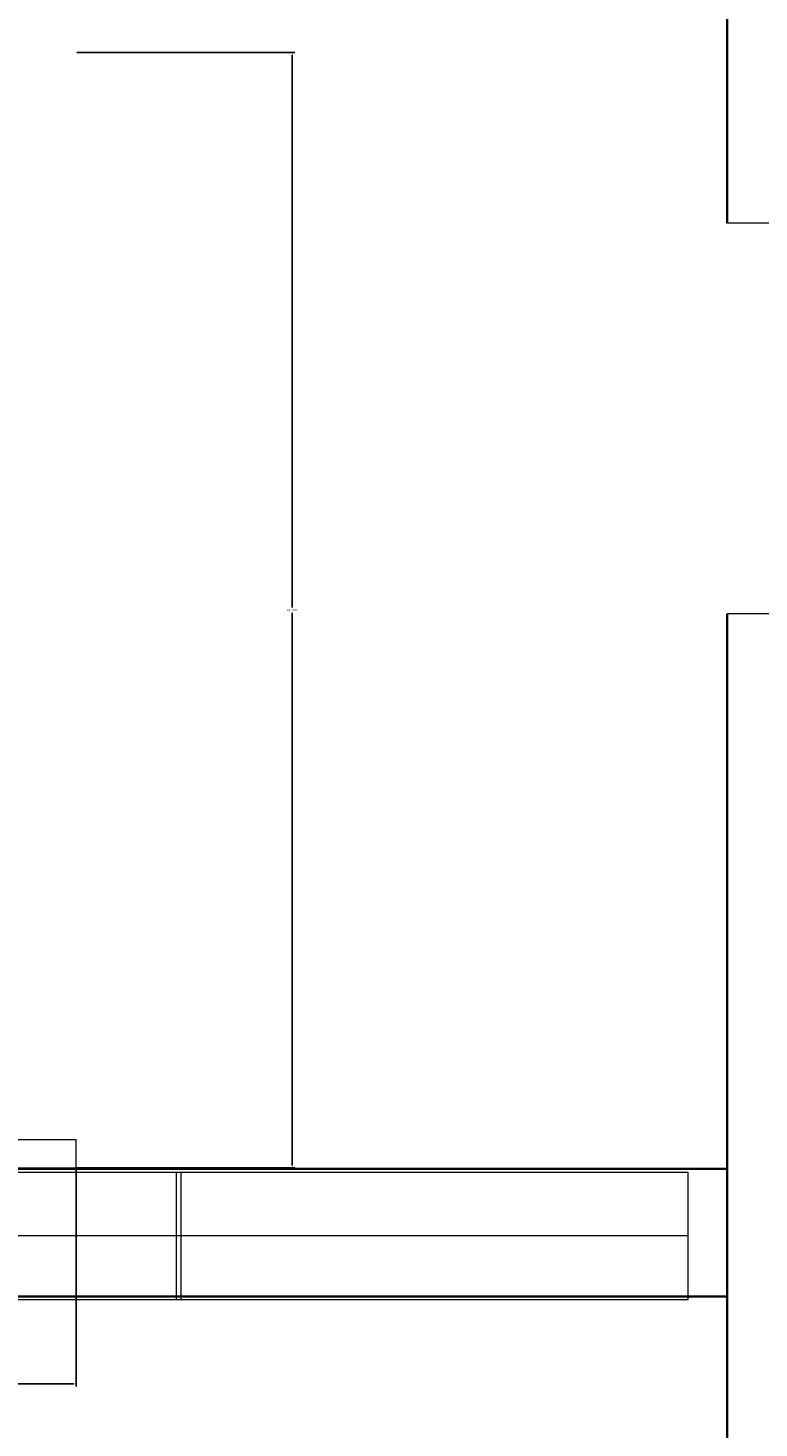
# Model space of a CAD drawing. Units: millimetres. Extents: x 27017497 to 27018854, y 7058029 to 7059154.
# Tile 27 of 91: x 27017753 to 27017804, y 7058124 to 7058222. Entities that reach past the tile are written whole.
import ezdxf

# ---------------------------------------------------------------- set-up
doc = ezdxf.new("R2010")
doc.units = ezdxf.units.MM
for name, color, linetype, lineweight in [('A-ANNO-DIMS', 2, 'Continuous', 18), ('A-DOOR', 4, 'Continuous', 20), ('A-FURN', 8, 'Continuous', 18), ('A-GLAZ', 4, 'Continuous', 18), ('A-WALL', 7, 'Continuous', 35)]:
    doc.layers.add(name, color=color, linetype=linetype, lineweight=lineweight)
doc.styles.get("Standard").update_dxf_attribs({"font": 'arial.ttf'})
doc.dimstyles.get("Standard").update_dxf_attribs({"dimtxt": 0.18, "dimasz": 0.18, "dimexe": 0.18, "dimexo": 0.0625, "dimgap": 0.09, "dimtad": 0, "dimtih": 1, "dimtoh": 1, "dimdec": 4, "dimzin": 0, "dimdsep": 46, "dimtxsty": 'Standard', "dimcen": 0.09, "dimadec": 0, "dimazin": 0, "dimtfac": 1, "dimtdec": 4, "dimtofl": 0, "dimtmove": 0, "dimatfit": 3, "dimfxl": 1, "dimtolj": 1, "dimtzin": 0, "dimarcsym": 0})

# ---------------------------------------------------------------- blocks, each defined once
blk = doc.blocks.new('*U2')
for p, q in [((0, 0), (0, -6)), ((40, 0), (40, -6))]:
    blk.add_line(p, q)
blk.add_lwpolyline([(0, 0), (0, 40), (1.75, 40), (1.75, 0)], close=True)
blk.add_arc((0, 0), 40, 0, 90)
blk = doc.blocks.new('CAMMAT')
for p, q in [((1.2731, 0), (-1.2731, 0)), ((-1.2731, 0), (-1.2731, -0.05)), ((1.2731, -0.05), (-1.2731, -0.05))]:
    blk.add_line(p, q)
blk = doc.blocks.new('WINDOW-SINGLE-LIGHT')
blk.add_lwpolyline([(36, 4.5), (36, 0), (0, 0), (0, 9), (36, 9), (36, 4.5), (0, 4.5)])
blk = doc.blocks.new('*D25')
at = {"layer": 'A-ANNO-DIMS', "color": 0, "lineweight": -2, "transparency": 16777216}
for p, q in [((27017654.932, 7058141.917), (27017654.932, 7058126.587)), ((27017756.349, 7058141.917), (27017756.349, 7058126.587)), ((27017655.112, 7058126.767), (27017704.753, 7058126.767)), ((27017756.169, 7058126.767), (27017706.528, 7058126.767))]:
    blk.add_line(p, q, dxfattribs=at)
at = {"layer": 'A-ANNO-DIMS', "color": 0, "transparency": 16777216}
for points in [[(27017655.112, 7058126.797), (27017655.112, 7058126.737), (27017654.932, 7058126.767)], [(27017756.169, 7058126.797), (27017756.169, 7058126.737), (27017756.349, 7058126.767)]]:
    blk.add_solid(points, dxfattribs=at)
at = {"layer": 'Defpoints', "color": 0, "transparency": 16777216}
for p in [(27017654.932, 7058141.98), (27017756.349, 7058141.98), (27017654.932, 7058126.767)]:
    blk.add_point(p, dxfattribs=at)
at = {"layer": 'A-ANNO-DIMS', "color": 0, "transparency": 16777216, "insert": (27017705.64, 7058126.767), "char_height": 0.18, "attachment_point": 5}
blk.add_mtext('\\A1;BED 101 TYP.', dxfattribs=at)
blk = doc.blocks.new('*D26')
at = {"layer": 'A-ANNO-DIMS', "color": 0, "lineweight": -2, "transparency": 16777216}
for p, q in [((27017756.412, 7058220.445), (27017771.742, 7058220.445)), ((27017771.562, 7058220.265), (27017771.562, 7058181.394)), ((27017771.562, 7058142.16), (27017771.562, 7058181.031)), ((27017756.412, 7058141.98), (27017771.742, 7058141.98))]:
    blk.add_line(p, q, dxfattribs=at)
at = {"layer": 'A-ANNO-DIMS', "color": 0, "transparency": 16777216}
for points in [[(27017771.532, 7058220.265), (27017771.592, 7058220.265), (27017771.562, 7058220.445)], [(27017771.532, 7058142.16), (27017771.592, 7058142.16), (27017771.562, 7058141.98)]]:
    blk.add_solid(points, dxfattribs=at)
at = {"layer": 'Defpoints', "color": 0, "transparency": 16777216}
for p in [(27017756.349, 7058220.445), (27017756.349, 7058141.98), (27017771.562, 7058141.98)]:
    blk.add_point(p, dxfattribs=at)
at = {"layer": 'A-ANNO-DIMS', "color": 0, "transparency": 16777216, "insert": (27017771.562, 7058181.212), "char_height": 0.18, "attachment_point": 5}
blk.add_mtext('\\A1;78 TYP.', dxfattribs=at)
blk = doc.blocks.new('*D47')
at = {"layer": 'A-ANNO-DIMS', "color": 0, "lineweight": -2, "transparency": 16777216}
for p, q in [((27017561.166, 7058294.35), (27017561.166, 7058028.6)), ((27018790.606, 7058294.35), (27018790.606, 7058028.6)), ((27017561.346, 7058028.78), (27018175.431, 7058028.78)), ((27018790.426, 7058028.78), (27018176.341, 7058028.78))]:
    blk.add_line(p, q, dxfattribs=at)
at = {"layer": 'A-ANNO-DIMS', "color": 0, "transparency": 16777216}
for points in [[(27017561.346, 7058028.81), (27017561.346, 7058028.75), (27017561.166, 7058028.78)], [(27018790.426, 7058028.81), (27018790.426, 7058028.75), (27018790.606, 7058028.78)]]:
    blk.add_solid(points, dxfattribs=at)
at = {"layer": 'Defpoints', "color": 0, "transparency": 16777216}
for p in [(27017561.166, 7058294.412), (27018790.606, 7058294.412), (27018790.606, 7058028.78)]:
    blk.add_point(p, dxfattribs=at)
at = {"layer": 'A-ANNO-DIMS', "color": 0, "transparency": 16777216, "insert": (27018175.886, 7058028.78), "char_height": 0.18, "attachment_point": 5}
blk.add_mtext('\\A1;1229.4', dxfattribs=at)
blk = doc.blocks.new('*D48')
at = {"layer": 'A-ANNO-DIMS', "color": 0, "lineweight": -2, "transparency": 16777216}
for p, q in [((27018463.498, 7058622.912), (27017497.536, 7058622.912)), ((27017497.716, 7058622.732), (27017497.716, 7058357.753)), ((27017497.716, 7058092.41), (27017497.716, 7058357.389)), ((27018555.129, 7058092.23), (27017497.536, 7058092.23))]:
    blk.add_line(p, q, dxfattribs=at)
at = {"layer": 'A-ANNO-DIMS', "color": 0, "transparency": 16777216}
for points in [[(27017497.686, 7058622.732), (27017497.746, 7058622.732), (27017497.716, 7058622.912)], [(27017497.686, 7058092.41), (27017497.746, 7058092.41), (27017497.716, 7058092.23)]]:
    blk.add_solid(points, dxfattribs=at)
at = {"layer": 'Defpoints', "color": 0, "transparency": 16777216}
for p in [(27018463.561, 7058622.912), (27017497.716, 7058092.23), (27018555.192, 7058092.23)]:
    blk.add_point(p, dxfattribs=at)
at = {"layer": 'A-ANNO-DIMS', "color": 0, "transparency": 16777216, "insert": (27017497.716, 7058357.571), "char_height": 0.18, "attachment_point": 5}
blk.add_mtext('\\A1;530.7', dxfattribs=at)

msp = doc.modelspace()

# ---------------------------------------------------------------- linework, layer by layer
at = {"layer": 'A-WALL'}
for p, q in [((27017802.166, 7058294.412), (27017802.166, 7058208.446)), ((27017802.166, 7058180.965), (27017802.166, 7058094.141)), ((27017622.666, 7058141.912), (27017802.166, 7058141.912)), ((27017613.666, 7058132.912), (27017802.166, 7058132.912)), ((27017613.666, 7058132.912), (27017802.166, 7058132.912))]:
    msp.add_line(p, q, dxfattribs=at)

# ---------------------------------------------------------------- block references
at = {"layer": 'A-DOOR', "xscale": 0.6870473523349573, "yscale": 0.6870473523349573, "zscale": 0.6870473523349573, "rotation": 270}
msp.add_blockref('*U2', (27017806.287, 7058208.446), dxfattribs=at)
at = {"layer": 'A-FURN', "xscale": 39.82996475819422, "yscale": 39.82996475819422, "zscale": 39.82996475819422, "rotation": 180}
msp.add_blockref('CAMMAT', (27017705.64, 7058141.98), dxfattribs=at)
at = {"layer": 'A-GLAZ'}
for p in [(27017727.724, 7058132.679), (27017763.411, 7058132.679)]:
    msp.add_blockref('WINDOW-SINGLE-LIGHT', p, dxfattribs=at)

# ---------------------------------------------------------------- dimensions: what is measured, and where the dimension line sits
at = {"layer": 'A-ANNO-DIMS'}
dim = msp.add_linear_dim(base=(27017497.716, 7058092.23), p1=(27018463.561, 7058622.912), p2=(27018555.192, 7058092.23), angle=90, dimstyle='Standard', override={"dimdec": 1, "dimlfac": 1, "dimrnd": 0, "dimzin": 0, "dimdsep": 46, "dimlunit": 2}, dxfattribs=at)
dim.commit()
dim.dimension.update_dxf_attribs({"geometry": '*D48', "text_midpoint": (27017497.716, 7058357.571)})
dim = msp.add_linear_dim(base=(27018790.606, 7058028.78), p1=(27017561.166, 7058294.412), p2=(27018790.606, 7058294.412), dimstyle='Standard', override={"dimdec": 1, "dimlfac": 1, "dimrnd": 0, "dimzin": 0, "dimdsep": 46, "dimlunit": 2}, dxfattribs=at)
dim.commit()
dim.dimension.update_dxf_attribs({"geometry": '*D47', "text_midpoint": (27018175.886, 7058028.78)})
for base, p1, p2, angle, text, picture, middle in [((27017771.562, 7058141.98), (27017756.349, 7058220.445), (27017756.349, 7058141.98), 270, '<> TYP.', '*D26', (27017771.562, 7058181.212)), ((27017654.932, 7058126.767), (27017756.349, 7058141.98), (27017654.932, 7058141.98), 180, 'BED <> TYP.', '*D25', (27017705.64, 7058126.767))]:
    dim = msp.add_linear_dim(base=base, p1=p1, p2=p2, angle=angle, text=text, dimstyle='Standard', override={"dimdec": 0, "dimlfac": 1, "dimrnd": 0, "dimzin": 0, "dimdsep": 46, "dimlunit": 2}, dxfattribs=at)
    dim.commit()
    dim.dimension.update_dxf_attribs({"geometry": picture, "text_midpoint": middle})

doc.saveas('drawing.dxf')
